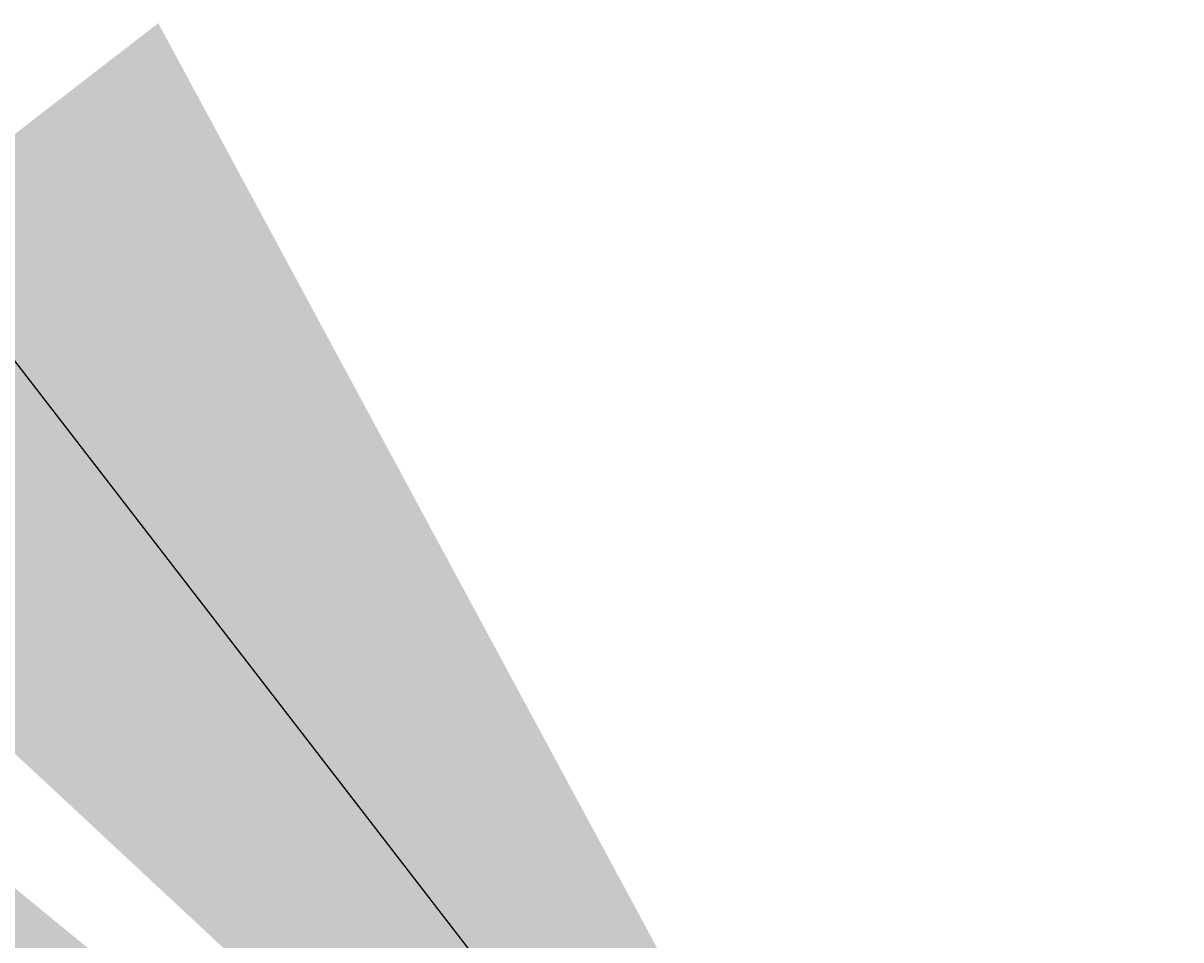
# Model space of a CAD drawing. Units: inches. Extents: x -9413 to 9703, y -9719 to 9096.
# Tile 1 of 1: x -5451 to 493, y 4393 to 9096. Entities that reach past the tile are written whole.
import ezdxf
from ezdxf import colors
from ezdxf.entities.mleader import LeaderData, LeaderLine
from ezdxf.math import Vec2, Vec3

# ---------------------------------------------------------------- set-up
doc = ezdxf.new("R2010")
doc.units = ezdxf.units.IN
doc.header["$MEASUREMENT"] = 0
doc.layers.add('M-ANNO-TEXT', color=7, linetype='Continuous', lineweight=18)
doc.styles.get("Standard").update_dxf_attribs({"font": 'arial.ttf'})

msp = doc.modelspace()

# ---------------------------------------------------------------- leaders
at = {"layer": 'M-ANNO-TEXT'}
ml = msp.add_multileader_mtext('Standard', dxfattribs=at)
ml.set_content('steam drum', color=256)
ml.set_leader_properties()
ml.build(insert=Vec2(0, 0))
ml.multileader.update_dxf_attribs({"dogleg_length": 0.36, "arrow_head_size": 10000, "scale": 10})
ctx = ml.context
ctx.base_point, ctx.scale, ctx.char_height, ctx.arrow_head_size, ctx.landing_gap_size, ctx.plane_origin = Vec3(1.078100315116472, 187.1657656808087), 10, 5.4, 10000, 0.9, Vec3(56.53630785249729, 178.1917761520126)
ctx.text_align_type = 2
notes = []
notes.append((ctx, [(0, (1, 1, 0), (49.60206616053652, 187.1657656808087), (-1, 0), 7.616326009130828, [(0, [(56.5363078524973, 178.1917761520126)], 0, [])])]))
ctx.mtext.insert, ctx.mtext.alignment, ctx.mtext.flow_direction = Vec3(41.08574015140569, 189.9099675907678), 3, 5
ml = msp.add_multileader_mtext('Standard', dxfattribs=at)
ml.set_content('Reheater', color=256)
ml.set_leader_properties()
ml.build(insert=Vec2(0, 0))
ml.multileader.update_dxf_attribs({"dogleg_length": 0.36, "arrow_head_size": 10000, "scale": 10})
ctx = ml.context
ctx.base_point, ctx.scale, ctx.char_height, ctx.arrow_head_size, ctx.landing_gap_size, ctx.plane_origin = Vec3(234.1414050860131, 159.7303554673012), 10, 5.4, 10000, 0.9, Vec3(221.1444910066821, 154.3050445940477)
notes.append((ctx, [(0, (1, 1, 0), (230.5414050860131, 159.7303554673012), (1, 0), 3.599999999999999, [(0, [(221.1444910066821, 154.3050445940477)], 0, [])])]))
ctx.mtext.insert, ctx.mtext.flow_direction = Vec3(235.0414050860131, 162.4745573772603), 5
ml = msp.add_multileader_mtext('Standard', dxfattribs=at)
ml.set_content('Boiler', color=256)
ml.set_leader_properties()
ml.build(insert=Vec2(0, 0))
ml.multileader.update_dxf_attribs({"dogleg_length": 0.36, "arrow_head_size": 10000, "scale": 10})
ctx = ml.context
ctx.base_point, ctx.scale, ctx.char_height, ctx.arrow_head_size, ctx.landing_gap_size, ctx.plane_origin = Vec3(31.04430257849453, 103.0991380116177), 10, 5.4, 10000, 0.9, Vec3(69.11352005531556, 99.3051261342938)
ctx.text_align_type = 2
notes.append((ctx, [(0, (1, 1, 0), (62.54209871927075, 103.0991380116177), (-1, 0), 10.86041551321825, [(0, [(69.11352005531556, 99.3051261342938)], 0, [])])]))
ctx.mtext.insert, ctx.mtext.alignment, ctx.mtext.flow_direction = Vec3(50.7816832060525, 105.8433399215768), 3, 5
for ctx, leaders in notes:
    for number, flags, end, landing, length, lines in leaders:
        leader = LeaderData()
        leader.index, (leader.has_last_leader_line, leader.has_dogleg_vector, leader.attachment_direction) = number, flags
        leader.last_leader_point, leader.dogleg_vector, leader.dogleg_length = Vec3(end), Vec3(landing), length
        for number, points, colour, breaks in lines:
            line = LeaderLine()
            line.index, line.vertices, line.color, line.breaks = number, Vec3.list(points), colors.encode_raw_color(colour), breaks
            leader.lines.append(line)
        ctx.leaders.append(leader)

doc.saveas('drawing.dxf')
